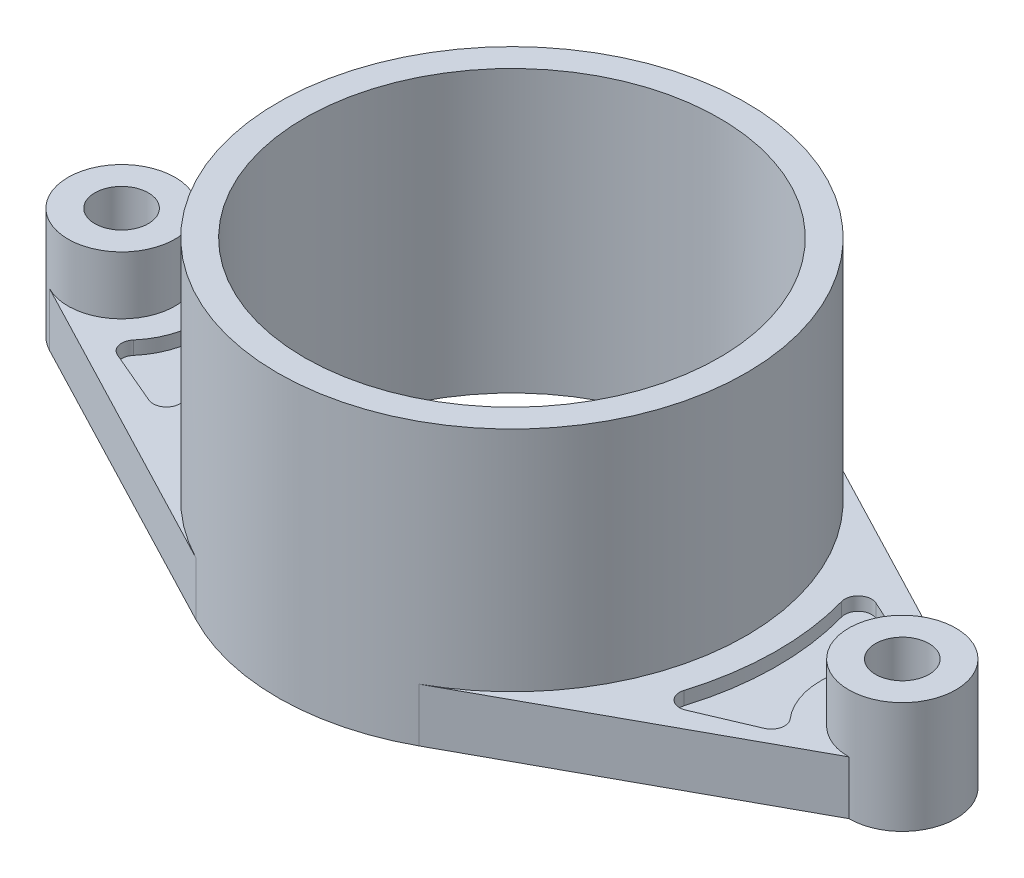
ISO-10303-21;
HEADER;
FILE_DESCRIPTION(('STEP AP214'),'2;1');
FILE_NAME('part.step','',(''),(''),'','','');
FILE_SCHEMA(('AUTOMOTIVE_DESIGN { 1 0 10303 214 1 1 1 1 }'));
ENDSEC;
DATA;
#1=APPLICATION_CONTEXT('core data for automotive mechanical design processes');
#2=APPLICATION_PROTOCOL_DEFINITION('international standard','automotive_design',2000,#1);
#3=PRODUCT_CONTEXT('',#1,'mechanical');
#4=PRODUCT('Part','Part','',(#3));
#5=PRODUCT_RELATED_PRODUCT_CATEGORY('part','',(#4));
#6=PRODUCT_DEFINITION_FORMATION('','',#4);
#7=PRODUCT_DEFINITION_CONTEXT('part definition',#1,'design');
#8=PRODUCT_DEFINITION('design','',#6,#7);
#9=PRODUCT_DEFINITION_SHAPE('','',#8);
#10=(LENGTH_UNIT() NAMED_UNIT(*) SI_UNIT(.MILLI.,.METRE.));
#11=(NAMED_UNIT(*) PLANE_ANGLE_UNIT() SI_UNIT($,.RADIAN.));
#12=(NAMED_UNIT(*) SI_UNIT($,.STERADIAN.) SOLID_ANGLE_UNIT());
#13=UNCERTAINTY_MEASURE_WITH_UNIT(LENGTH_MEASURE(1.E-05),#10,'distance_accuracy_value','');
#14=(GEOMETRIC_REPRESENTATION_CONTEXT(3) GLOBAL_UNCERTAINTY_ASSIGNED_CONTEXT((#13)) GLOBAL_UNIT_ASSIGNED_CONTEXT((#10,
#11,#12)) REPRESENTATION_CONTEXT('',''));
#15=CARTESIAN_POINT('',(0.,0.,0.));
#16=DIRECTION('',(0.,0.,1.));
#17=DIRECTION('',(1.,0.,0.));
#18=AXIS2_PLACEMENT_3D('',#15,#16,#17);
#19=CARTESIAN_POINT('',(0.,12.,0.));
#20=DIRECTION('',(0.,1.,0.));
#21=DIRECTION('',(0.,0.,1.));
#22=AXIS2_PLACEMENT_3D('',#19,#20,#21);
#23=PLANE('',#22);
#24=CARTESIAN_POINT('',(87.5,12.,0.));
#25=DIRECTION('',(0.,1.,0.));
#26=DIRECTION('',(0.,0.,1.));
#27=AXIS2_PLACEMENT_3D('',#24,#25,#26);
#28=CIRCLE('',#27,12.);
#29=CARTESIAN_POINT('',(93.0542857142854,12.,-10.6371946585583));
#30=VERTEX_POINT('',#29);
#31=CARTESIAN_POINT('',(87.5,12.,12.));
#32=VERTEX_POINT('',#31);
#33=EDGE_CURVE('E362',#30,#32,#28,.T.);
#34=ORIENTED_EDGE('',*,*,#33,.F.);
#35=DIRECTION('',(-0.886432888213266,0.,-0.462857142857154));
#36=VECTOR('',#35,1.);
#37=CARTESIAN_POINT('',(24.3000000000006,12.,-46.5377266311965));
#38=LINE('',#37,#36);
#39=CARTESIAN_POINT('',(24.3000000000006,12.,-46.5377266311965));
#40=VERTEX_POINT('',#39);
#41=EDGE_CURVE('E364',#30,#40,#38,.T.);
#42=ORIENTED_EDGE('',*,*,#41,.T.);
#43=CARTESIAN_POINT('',(0.,12.,0.));
#44=DIRECTION('',(0.,1.,0.));
#45=DIRECTION('',(0.,0.,1.));
#46=AXIS2_PLACEMENT_3D('',#43,#44,#45);
#47=CIRCLE('',#46,52.5);
#48=CARTESIAN_POINT('',(25.1823425044712,12.,46.0662525715681));
#49=VERTEX_POINT('',#48);
#50=EDGE_CURVE('E369',#49,#40,#47,.T.);
#51=ORIENTED_EDGE('',*,*,#50,.F.);
#52=DIRECTION('',(-0.877452429934631,0.,0.479663666751831));
#53=VECTOR('',#52,1.);
#54=CARTESIAN_POINT('',(25.1823425044711,12.,46.0662525715681));
#55=LINE('',#54,#53);
#56=EDGE_CURVE('E371',#32,#49,#55,.T.);
#57=ORIENTED_EDGE('',*,*,#56,.F.);
#58=EDGE_LOOP('',(#34,#42,#51,#57));
#59=FACE_BOUND('',#58,.T.);
#60=CARTESIAN_POINT('',(59.4229736389567,12.,-18.1878630690945));
#61=DIRECTION('',(0.,1.,0.));
#62=DIRECTION('',(0.,0.,-1.));
#63=AXIS2_PLACEMENT_3D('',#60,#61,#62);
#64=CIRCLE('',#63,3.);
#65=CARTESIAN_POINT('',(60.670465140095,12.,-20.9161894708631));
#66=VERTEX_POINT('',#65);
#67=CARTESIAN_POINT('',(56.5356423498588,12.,-17.3734196843239));
#68=VERTEX_POINT('',#67);
#69=EDGE_CURVE('E69',#66,#68,#64,.T.);
#70=ORIENTED_EDGE('',*,*,#69,.F.);
#71=DIRECTION('',(-0.90944213392287,0.,-0.415830500379442));
#72=VECTOR('',#71,1.);
#73=CARTESIAN_POINT('',(60.670465140095,12.,-20.9161894708631));
#74=LINE('',#73,#72);
#75=CARTESIAN_POINT('',(72.8322479303877,12.,-15.3553736316198));
#76=VERTEX_POINT('',#75);
#77=EDGE_CURVE('E278',#76,#66,#74,.T.);
#78=ORIENTED_EDGE('',*,*,#77,.F.);
#79=CARTESIAN_POINT('',(71.5847564292494,12.,-12.6270472298512));
#80=DIRECTION('',(0.,1.,0.));
#81=DIRECTION('',(0.,0.,-1.));
#82=AXIS2_PLACEMENT_3D('',#79,#80,#81);
#83=CIRCLE('',#82,3.);
#84=CARTESIAN_POINT('',(73.8195893160945,12.,-10.6256672139932));
#85=VERTEX_POINT('',#84);
#86=EDGE_CURVE('E318',#85,#76,#83,.T.);
#87=ORIENTED_EDGE('',*,*,#86,.F.);
#88=CARTESIAN_POINT('',(86.1725998126227,12.,0.436935492886657));
#89=DIRECTION('',(0.,-1.,0.));
#90=DIRECTION('',(0.,0.,1.));
#91=AXIS2_PLACEMENT_3D('',#88,#89,#90);
#92=CIRCLE('',#91,16.5824620300365);
#93=CARTESIAN_POINT('',(73.5829785567061,12.,11.2295016200955));
#94=VERTEX_POINT('',#93);
#95=EDGE_CURVE('E312',#94,#85,#92,.T.);
#96=ORIENTED_EDGE('',*,*,#95,.F.);
#97=CARTESIAN_POINT('',(71.3053394643122,12.,13.1820282306181));
#98=DIRECTION('',(0.,1.,0.));
#99=DIRECTION('',(0.,0.,-1.));
#100=AXIS2_PLACEMENT_3D('',#97,#98,#99);
#101=CIRCLE('',#100,3.);
#102=CARTESIAN_POINT('',(72.4819315608604,12.,15.941671511613));
#103=VERTEX_POINT('',#102);
#104=EDGE_CURVE('E315',#103,#94,#101,.T.);
#105=ORIENTED_EDGE('',*,*,#104,.F.);
#106=DIRECTION('',(0.919881093664966,0.,-0.392197365516071));
#107=VECTOR('',#106,1.);
#108=CARTESIAN_POINT('',(60.1771351937797,12.,21.1879025208334));
#109=LINE('',#108,#107);
#110=CARTESIAN_POINT('',(60.1771351937797,12.,21.1879025208334));
#111=VERTEX_POINT('',#110);
#112=EDGE_CURVE('E310',#111,#103,#109,.T.);
#113=ORIENTED_EDGE('',*,*,#112,.F.);
#114=CARTESIAN_POINT('',(59.0005430972315,12.,18.4282592398385));
#115=DIRECTION('',(0.,1.,0.));
#116=DIRECTION('',(0.,0.,-1.));
#117=AXIS2_PLACEMENT_3D('',#114,#115,#116);
#118=CIRCLE('',#117,3.);
#119=CARTESIAN_POINT('',(56.1327698280164,12.,17.5474207322928));
#120=VERTEX_POINT('',#119);
#121=EDGE_CURVE('E308',#120,#111,#118,.T.);
#122=ORIENTED_EDGE('',*,*,#121,.F.);
#123=CARTESIAN_POINT('',(-2.94003283636643,12.,-0.596830730682654));
#124=DIRECTION('',(0.,-1.,0.));
#125=DIRECTION('',(0.,0.,-1.));
#126=AXIS2_PLACEMENT_3D('',#123,#124,#125);
#127=CIRCLE('',#126,61.7965199325723);
#128=EDGE_CURVE('E305',#68,#120,#127,.T.);
#129=ORIENTED_EDGE('',*,*,#128,.F.);
#130=EDGE_LOOP('',(#70,#78,#87,#96,#105,#113,#122,#129));
#131=FACE_BOUND('',#130,.T.);
#132=ADVANCED_FACE('F41',(#59,#131),#23,.T.);
#133=CARTESIAN_POINT('',(0.,63.,0.));
#134=DIRECTION('',(0.,-1.,0.));
#135=DIRECTION('',(0.,0.,-1.));
#136=AXIS2_PLACEMENT_3D('',#133,#134,#135);
#137=CYLINDRICAL_SURFACE('',#136,52.5);
#138=ORIENTED_EDGE('',*,*,#50,.T.);
#139=DIRECTION('',(0.,-1.,0.));
#140=VECTOR('',#139,1.);
#141=CARTESIAN_POINT('',(24.3000000000006,12.,-46.5377266311965));
#142=LINE('',#141,#140);
#143=CARTESIAN_POINT('',(24.3000000000006,0.,-46.5377266311965));
#144=VERTEX_POINT('',#143);
#145=EDGE_CURVE('E383',#40,#144,#142,.T.);
#146=ORIENTED_EDGE('',*,*,#145,.T.);
#147=CARTESIAN_POINT('',(0.,0.,0.));
#148=DIRECTION('',(0.,1.,0.));
#149=DIRECTION('',(0.,0.,1.));
#150=AXIS2_PLACEMENT_3D('',#147,#148,#149);
#151=CIRCLE('',#150,52.5);
#152=CARTESIAN_POINT('',(-24.3000000000006,0.,-46.5377266311965));
#153=VERTEX_POINT('',#152);
#154=EDGE_CURVE('E418',#144,#153,#151,.T.);
#155=ORIENTED_EDGE('',*,*,#154,.T.);
#156=DIRECTION('',(0.,-1.,0.));
#157=VECTOR('',#156,1.);
#158=CARTESIAN_POINT('',(-24.3000000000006,12.,-46.5377266311965));
#159=LINE('',#158,#157);
#160=CARTESIAN_POINT('',(-24.3000000000006,12.,-46.5377266311965));
#161=VERTEX_POINT('',#160);
#162=EDGE_CURVE('E413',#161,#153,#159,.T.);
#163=ORIENTED_EDGE('',*,*,#162,.F.);
#164=CARTESIAN_POINT('',(0.,12.,0.));
#165=DIRECTION('',(0.,1.,0.));
#166=DIRECTION('',(0.,0.,1.));
#167=AXIS2_PLACEMENT_3D('',#164,#165,#166);
#168=CIRCLE('',#167,52.5);
#169=CARTESIAN_POINT('',(-24.3000000000006,12.,46.5377266311965));
#170=VERTEX_POINT('',#169);
#171=EDGE_CURVE('E388',#161,#170,#168,.T.);
#172=ORIENTED_EDGE('',*,*,#171,.T.);
#173=DIRECTION('',(0.,-1.,0.));
#174=VECTOR('',#173,1.);
#175=CARTESIAN_POINT('',(-24.3000000000006,12.,46.5377266311965));
#176=LINE('',#175,#174);
#177=CARTESIAN_POINT('',(-24.3000000000006,0.,46.5377266311965));
#178=VERTEX_POINT('',#177);
#179=EDGE_CURVE('E405',#170,#178,#176,.T.);
#180=ORIENTED_EDGE('',*,*,#179,.T.);
#181=CARTESIAN_POINT('',(25.1823425044712,0.,46.0662525715681));
#182=VERTEX_POINT('',#181);
#183=EDGE_CURVE('E49',#178,#182,#151,.T.);
#184=ORIENTED_EDGE('',*,*,#183,.T.);
#185=DIRECTION('',(0.,-1.,0.));
#186=VECTOR('',#185,1.);
#187=CARTESIAN_POINT('',(25.1823425044711,12.,46.0662525715681));
#188=LINE('',#187,#186);
#189=EDGE_CURVE('E381',#49,#182,#188,.T.);
#190=ORIENTED_EDGE('',*,*,#189,.F.);
#191=EDGE_LOOP('',(#138,#146,#155,#163,#172,#180,#184,#190));
#192=FACE_BOUND('',#191,.T.);
#193=CARTESIAN_POINT('',(0.,63.,0.));
#194=DIRECTION('',(0.,1.,0.));
#195=DIRECTION('',(0.,0.,1.));
#196=AXIS2_PLACEMENT_3D('',#193,#194,#195);
#197=CIRCLE('',#196,52.5);
#198=CARTESIAN_POINT('',(0.,63.,52.5));
#199=VERTEX_POINT('',#198);
#200=EDGE_CURVE('E11',#199,#199,#197,.T.);
#201=ORIENTED_EDGE('',*,*,#200,.F.);
#202=EDGE_LOOP('',(#201));
#203=FACE_BOUND('',#202,.T.);
#204=ADVANCED_FACE('F43',(#192,#203),#137,.T.);
#205=CARTESIAN_POINT('',(0.,63.,0.));
#206=DIRECTION('',(0.,1.,0.));
#207=DIRECTION('',(0.,0.,1.));
#208=AXIS2_PLACEMENT_3D('',#205,#206,#207);
#209=PLANE('',#208);
#210=CARTESIAN_POINT('',(0.,63.,0.));
#211=DIRECTION('',(0.,1.,0.));
#212=DIRECTION('',(0.,0.,1.));
#213=AXIS2_PLACEMENT_3D('',#210,#211,#212);
#214=CIRCLE('',#213,46.5);
#215=CARTESIAN_POINT('',(0.,63.,46.5));
#216=VERTEX_POINT('',#215);
#217=EDGE_CURVE('E343',#216,#216,#214,.T.);
#218=ORIENTED_EDGE('',*,*,#217,.F.);
#219=EDGE_LOOP('',(#218));
#220=FACE_BOUND('',#219,.T.);
#221=ORIENTED_EDGE('',*,*,#200,.T.);
#222=EDGE_LOOP('',(#221));
#223=FACE_BOUND('',#222,.T.);
#224=ADVANCED_FACE('F486',(#220,#223),#209,.T.);
#225=CARTESIAN_POINT('',(0.,0.,0.));
#226=DIRECTION('',(0.,1.,0.));
#227=DIRECTION('',(0.,0.,1.));
#228=AXIS2_PLACEMENT_3D('',#225,#226,#227);
#229=PLANE('',#228);
#230=CARTESIAN_POINT('',(-87.5,0.,0.));
#231=DIRECTION('',(0.,1.,0.));
#232=DIRECTION('',(0.,0.,1.));
#233=AXIS2_PLACEMENT_3D('',#230,#231,#232);
#234=CIRCLE('',#233,6.);
#235=CARTESIAN_POINT('',(-87.5,0.,6.));
#236=VERTEX_POINT('',#235);
#237=EDGE_CURVE('E339',#236,#236,#234,.T.);
#238=ORIENTED_EDGE('',*,*,#237,.T.);
#239=EDGE_LOOP('',(#238));
#240=FACE_BOUND('',#239,.T.);
#241=CARTESIAN_POINT('',(0.,0.,0.));
#242=DIRECTION('',(0.,1.,0.));
#243=DIRECTION('',(0.,0.,1.));
#244=AXIS2_PLACEMENT_3D('',#241,#242,#243);
#245=CIRCLE('',#244,46.5);
#246=CARTESIAN_POINT('',(0.,0.,46.5));
#247=VERTEX_POINT('',#246);
#248=EDGE_CURVE('E344',#247,#247,#245,.T.);
#249=ORIENTED_EDGE('',*,*,#248,.T.);
#250=EDGE_LOOP('',(#249));
#251=FACE_BOUND('',#250,.T.);
#252=CARTESIAN_POINT('',(87.5,0.,0.));
#253=DIRECTION('',(0.,1.,0.));
#254=DIRECTION('',(0.,0.,1.));
#255=AXIS2_PLACEMENT_3D('',#252,#253,#254);
#256=CIRCLE('',#255,6.);
#257=CARTESIAN_POINT('',(87.5,0.,6.));
#258=VERTEX_POINT('',#257);
#259=EDGE_CURVE('E262',#258,#258,#256,.T.);
#260=ORIENTED_EDGE('',*,*,#259,.T.);
#261=EDGE_LOOP('',(#260));
#262=FACE_BOUND('',#261,.T.);
#263=ORIENTED_EDGE('',*,*,#183,.F.);
#264=DIRECTION('',(0.886432888213266,0.,0.462857142857154));
#265=VECTOR('',#264,1.);
#266=CARTESIAN_POINT('',(-24.3000000000006,0.,46.5377266311965));
#267=LINE('',#266,#265);
#268=CARTESIAN_POINT('',(-93.0542857142854,0.,10.6371946585583));
#269=VERTEX_POINT('',#268);
#270=EDGE_CURVE('E395',#269,#178,#267,.T.);
#271=ORIENTED_EDGE('',*,*,#270,.F.);
#272=CARTESIAN_POINT('',(-87.5,0.,0.));
#273=DIRECTION('',(0.,1.,0.));
#274=DIRECTION('',(0.,0.,1.));
#275=AXIS2_PLACEMENT_3D('',#272,#273,#274);
#276=CIRCLE('',#275,12.);
#277=CARTESIAN_POINT('',(-93.0542857142854,0.,-10.6371946585583));
#278=VERTEX_POINT('',#277);
#279=EDGE_CURVE('E349',#278,#269,#276,.T.);
#280=ORIENTED_EDGE('',*,*,#279,.F.);
#281=DIRECTION('',(0.886432888213266,0.,-0.462857142857154));
#282=VECTOR('',#281,1.);
#283=CARTESIAN_POINT('',(-24.3000000000006,0.,-46.5377266311965));
#284=LINE('',#283,#282);
#285=EDGE_CURVE('E386',#278,#153,#284,.T.);
#286=ORIENTED_EDGE('',*,*,#285,.T.);
#287=ORIENTED_EDGE('',*,*,#154,.F.);
#288=DIRECTION('',(-0.886432888213266,0.,-0.462857142857154));
#289=VECTOR('',#288,1.);
#290=CARTESIAN_POINT('',(24.3000000000006,0.,-46.5377266311965));
#291=LINE('',#290,#289);
#292=CARTESIAN_POINT('',(93.0542857142854,0.,-10.6371946585583));
#293=VERTEX_POINT('',#292);
#294=EDGE_CURVE('E358',#293,#144,#291,.T.);
#295=ORIENTED_EDGE('',*,*,#294,.F.);
#296=CARTESIAN_POINT('',(87.5,0.,0.));
#297=DIRECTION('',(0.,1.,0.));
#298=DIRECTION('',(0.,0.,1.));
#299=AXIS2_PLACEMENT_3D('',#296,#297,#298);
#300=CIRCLE('',#299,12.);
#301=CARTESIAN_POINT('',(87.5,0.,11.9999999999991));
#302=VERTEX_POINT('',#301);
#303=EDGE_CURVE('E354',#302,#293,#300,.T.);
#304=ORIENTED_EDGE('',*,*,#303,.F.);
#305=DIRECTION('',(-0.877452429934631,0.,0.479663666751831));
#306=VECTOR('',#305,1.);
#307=CARTESIAN_POINT('',(25.1823425044711,0.,46.0662525715681));
#308=LINE('',#307,#306);
#309=EDGE_CURVE('E368',#302,#182,#308,.T.);
#310=ORIENTED_EDGE('',*,*,#309,.T.);
#311=EDGE_LOOP('',(#263,#271,#280,#286,#287,#295,#304,#310));
#312=FACE_BOUND('',#311,.T.);
#313=ADVANCED_FACE('F441',(#240,#251,#262,#312),#229,.F.);
#314=CARTESIAN_POINT('',(-24.3000000000006,12.,-46.5377266311965));
#315=DIRECTION('',(-0.462857142857154,0.,-0.886432888213266));
#316=DIRECTION('',(-0.886432888213266,0.,0.462857142857154));
#317=AXIS2_PLACEMENT_3D('',#314,#315,#316);
#318=PLANE('',#317);
#319=ORIENTED_EDGE('',*,*,#285,.F.);
#320=DIRECTION('',(0.,-1.,0.));
#321=VECTOR('',#320,1.);
#322=CARTESIAN_POINT('',(-93.0542857142854,12.,-10.6371946585583));
#323=LINE('',#322,#321);
#324=CARTESIAN_POINT('',(-93.0542857142854,12.,-10.6371946585583));
#325=VERTEX_POINT('',#324);
#326=EDGE_CURVE('E414',#325,#278,#323,.T.);
#327=ORIENTED_EDGE('',*,*,#326,.F.);
#328=DIRECTION('',(0.886432888213266,0.,-0.462857142857154));
#329=VECTOR('',#328,1.);
#330=CARTESIAN_POINT('',(-24.3000000000006,12.,-46.5377266311965));
#331=LINE('',#330,#329);
#332=EDGE_CURVE('E394',#325,#161,#331,.T.);
#333=ORIENTED_EDGE('',*,*,#332,.T.);
#334=ORIENTED_EDGE('',*,*,#162,.T.);
#335=EDGE_LOOP('',(#319,#327,#333,#334));
#336=FACE_BOUND('',#335,.T.);
#337=ADVANCED_FACE('F463',(#336),#318,.T.);
#338=CARTESIAN_POINT('',(-24.3000000000006,12.,46.5377266311965));
#339=DIRECTION('',(0.462857142857154,0.,-0.886432888213266));
#340=DIRECTION('',(-0.886432888213266,0.,-0.462857142857154));
#341=AXIS2_PLACEMENT_3D('',#338,#339,#340);
#342=PLANE('',#341);
#343=ORIENTED_EDGE('',*,*,#270,.T.);
#344=ORIENTED_EDGE('',*,*,#179,.F.);
#345=DIRECTION('',(0.886432888213266,0.,0.462857142857154));
#346=VECTOR('',#345,1.);
#347=CARTESIAN_POINT('',(-24.3000000000006,12.,46.5377266311965));
#348=LINE('',#347,#346);
#349=CARTESIAN_POINT('',(-93.0542857142854,12.,10.6371946585583));
#350=VERTEX_POINT('',#349);
#351=EDGE_CURVE('E398',#350,#170,#348,.T.);
#352=ORIENTED_EDGE('',*,*,#351,.F.);
#353=DIRECTION('',(0.,-1.,0.));
#354=VECTOR('',#353,1.);
#355=CARTESIAN_POINT('',(-93.0542857142854,12.,10.6371946585583));
#356=LINE('',#355,#354);
#357=EDGE_CURVE('E406',#350,#269,#356,.T.);
#358=ORIENTED_EDGE('',*,*,#357,.T.);
#359=EDGE_LOOP('',(#343,#344,#352,#358));
#360=FACE_BOUND('',#359,.T.);
#361=ADVANCED_FACE('F468',(#360),#342,.F.);
#362=CARTESIAN_POINT('',(0.,12.,0.));
#363=DIRECTION('',(0.,1.,0.));
#364=DIRECTION('',(0.,0.,1.));
#365=AXIS2_PLACEMENT_3D('',#362,#363,#364);
#366=PLANE('',#365);
#367=CARTESIAN_POINT('',(-71.3053394643122,12.,13.1820282306181));
#368=DIRECTION('',(0.,1.,0.));
#369=DIRECTION('',(0.,0.,1.));
#370=AXIS2_PLACEMENT_3D('',#367,#368,#369);
#371=CIRCLE('',#370,3.);
#372=CARTESIAN_POINT('',(-73.5829785567061,12.,11.2295016200955));
#373=VERTEX_POINT('',#372);
#374=CARTESIAN_POINT('',(-72.4819315608604,12.,15.941671511613));
#375=VERTEX_POINT('',#374);
#376=EDGE_CURVE('E59',#373,#375,#371,.T.);
#377=ORIENTED_EDGE('',*,*,#376,.F.);
#378=CARTESIAN_POINT('',(-86.1725998126227,12.,0.436935492886657));
#379=DIRECTION('',(0.,-1.,0.));
#380=DIRECTION('',(0.,0.,-1.));
#381=AXIS2_PLACEMENT_3D('',#378,#379,#380);
#382=CIRCLE('',#381,16.5824620300365);
#383=CARTESIAN_POINT('',(-73.8195893160945,12.,-10.6256672139932));
#384=VERTEX_POINT('',#383);
#385=EDGE_CURVE('E223',#384,#373,#382,.T.);
#386=ORIENTED_EDGE('',*,*,#385,.F.);
#387=CARTESIAN_POINT('',(-71.5847564292494,12.,-12.6270472298512));
#388=DIRECTION('',(0.,1.,0.));
#389=DIRECTION('',(0.,0.,1.));
#390=AXIS2_PLACEMENT_3D('',#387,#388,#389);
#391=CIRCLE('',#390,3.);
#392=CARTESIAN_POINT('',(-72.8322479303877,12.,-15.3553736316198));
#393=VERTEX_POINT('',#392);
#394=EDGE_CURVE('E230',#393,#384,#391,.T.);
#395=ORIENTED_EDGE('',*,*,#394,.F.);
#396=DIRECTION('',(-0.90944213392287,0.,0.415830500379442));
#397=VECTOR('',#396,1.);
#398=CARTESIAN_POINT('',(-60.670465140095,12.,-20.9161894708631));
#399=LINE('',#398,#397);
#400=CARTESIAN_POINT('',(-60.670465140095,12.,-20.9161894708631));
#401=VERTEX_POINT('',#400);
#402=EDGE_CURVE('E260',#401,#393,#399,.T.);
#403=ORIENTED_EDGE('',*,*,#402,.F.);
#404=CARTESIAN_POINT('',(-59.4229736389567,12.,-18.1878630690945));
#405=DIRECTION('',(0.,1.,0.));
#406=DIRECTION('',(0.,0.,1.));
#407=AXIS2_PLACEMENT_3D('',#404,#405,#406);
#408=CIRCLE('',#407,3.);
#409=CARTESIAN_POINT('',(-56.5356423498588,12.,-17.3734196843239));
#410=VERTEX_POINT('',#409);
#411=EDGE_CURVE('E255',#410,#401,#408,.T.);
#412=ORIENTED_EDGE('',*,*,#411,.F.);
#413=CARTESIAN_POINT('',(2.94003283636643,12.,-0.596830730682654));
#414=DIRECTION('',(0.,-1.,0.));
#415=DIRECTION('',(0.,0.,1.));
#416=AXIS2_PLACEMENT_3D('',#413,#414,#415);
#417=CIRCLE('',#416,61.7965199325723);
#418=CARTESIAN_POINT('',(-56.1327698280164,12.,17.5474207322928));
#419=VERTEX_POINT('',#418);
#420=EDGE_CURVE('E253',#419,#410,#417,.T.);
#421=ORIENTED_EDGE('',*,*,#420,.F.);
#422=CARTESIAN_POINT('',(-59.0005430972315,12.,18.4282592398385));
#423=DIRECTION('',(0.,1.,0.));
#424=DIRECTION('',(0.,0.,1.));
#425=AXIS2_PLACEMENT_3D('',#422,#423,#424);
#426=CIRCLE('',#425,2.99999999999997);
#427=CARTESIAN_POINT('',(-60.1771351937798,12.,21.1879025208334));
#428=VERTEX_POINT('',#427);
#429=EDGE_CURVE('E250',#428,#419,#426,.T.);
#430=ORIENTED_EDGE('',*,*,#429,.F.);
#431=DIRECTION('',(0.919881093664967,0.,0.392197365516067));
#432=VECTOR('',#431,1.);
#433=CARTESIAN_POINT('',(-60.1771351937797,12.,21.1879025208334));
#434=LINE('',#433,#432);
#435=EDGE_CURVE('E243',#375,#428,#434,.T.);
#436=ORIENTED_EDGE('',*,*,#435,.F.);
#437=EDGE_LOOP('',(#377,#386,#395,#403,#412,#421,#430,#436));
#438=FACE_BOUND('',#437,.T.);
#439=ORIENTED_EDGE('',*,*,#171,.F.);
#440=ORIENTED_EDGE('',*,*,#332,.F.);
#441=CARTESIAN_POINT('',(-87.5,12.,0.));
#442=DIRECTION('',(0.,1.,0.));
#443=DIRECTION('',(0.,0.,1.));
#444=AXIS2_PLACEMENT_3D('',#441,#442,#443);
#445=CIRCLE('',#444,12.);
#446=EDGE_CURVE('E399',#350,#325,#445,.T.);
#447=ORIENTED_EDGE('',*,*,#446,.F.);
#448=ORIENTED_EDGE('',*,*,#351,.T.);
#449=EDGE_LOOP('',(#439,#440,#447,#448));
#450=FACE_BOUND('',#449,.T.);
#451=ADVANCED_FACE('F470',(#438,#450),#366,.T.);
#452=CARTESIAN_POINT('',(24.3000000000006,12.,-46.5377266311965));
#453=DIRECTION('',(-0.462857142857154,0.,0.886432888213266));
#454=DIRECTION('',(0.886432888213266,0.,0.462857142857154));
#455=AXIS2_PLACEMENT_3D('',#452,#453,#454);
#456=PLANE('',#455);
#457=ORIENTED_EDGE('',*,*,#294,.T.);
#458=ORIENTED_EDGE('',*,*,#145,.F.);
#459=ORIENTED_EDGE('',*,*,#41,.F.);
#460=DIRECTION('',(0.,-1.,0.));
#461=VECTOR('',#460,1.);
#462=CARTESIAN_POINT('',(93.0542857142854,12.,-10.6371946585583));
#463=LINE('',#462,#461);
#464=EDGE_CURVE('E390',#30,#293,#463,.T.);
#465=ORIENTED_EDGE('',*,*,#464,.T.);
#466=EDGE_LOOP('',(#457,#458,#459,#465));
#467=FACE_BOUND('',#466,.T.);
#468=ADVANCED_FACE('F449',(#467),#456,.F.);
#469=CARTESIAN_POINT('',(25.1823425044711,12.,46.0662525715681));
#470=DIRECTION('',(0.479663666751831,0.,0.877452429934631));
#471=DIRECTION('',(0.877452429934631,0.,-0.479663666751831));
#472=AXIS2_PLACEMENT_3D('',#469,#470,#471);
#473=PLANE('',#472);
#474=ORIENTED_EDGE('',*,*,#309,.F.);
#475=DIRECTION('',(0.,-1.,0.));
#476=VECTOR('',#475,1.);
#477=CARTESIAN_POINT('',(87.5,12.,11.9999999999991));
#478=LINE('',#477,#476);
#479=EDGE_CURVE('E372',#32,#302,#478,.T.);
#480=ORIENTED_EDGE('',*,*,#479,.F.);
#481=ORIENTED_EDGE('',*,*,#56,.T.);
#482=ORIENTED_EDGE('',*,*,#189,.T.);
#483=EDGE_LOOP('',(#474,#480,#481,#482));
#484=FACE_BOUND('',#483,.T.);
#485=ADVANCED_FACE('F440',(#484),#473,.T.);
#486=CARTESIAN_POINT('',(87.5,25.,0.));
#487=DIRECTION('',(0.,-1.,0.));
#488=DIRECTION('',(0.,0.,-1.));
#489=AXIS2_PLACEMENT_3D('',#486,#487,#488);
#490=CYLINDRICAL_SURFACE('',#489,12.);
#491=CARTESIAN_POINT('',(87.5,25.,0.));
#492=DIRECTION('',(0.,1.,0.));
#493=DIRECTION('',(0.,0.,1.));
#494=AXIS2_PLACEMENT_3D('',#491,#492,#493);
#495=CIRCLE('',#494,12.);
#496=CARTESIAN_POINT('',(87.5,25.,12.));
#497=VERTEX_POINT('',#496);
#498=EDGE_CURVE('E359',#497,#497,#495,.T.);
#499=ORIENTED_EDGE('',*,*,#498,.F.);
#500=EDGE_LOOP('',(#499));
#501=FACE_BOUND('',#500,.T.);
#502=ORIENTED_EDGE('',*,*,#303,.T.);
#503=ORIENTED_EDGE('',*,*,#464,.F.);
#504=ORIENTED_EDGE('',*,*,#33,.T.);
#505=ORIENTED_EDGE('',*,*,#479,.T.);
#506=EDGE_LOOP('',(#502,#503,#504,#505));
#507=FACE_BOUND('',#506,.T.);
#508=ADVANCED_FACE('F431',(#501,#507),#490,.T.);
#509=CARTESIAN_POINT('',(0.,25.,0.));
#510=DIRECTION('',(0.,1.,0.));
#511=DIRECTION('',(0.,0.,1.));
#512=AXIS2_PLACEMENT_3D('',#509,#510,#511);
#513=PLANE('',#512);
#514=CARTESIAN_POINT('',(87.5,25.,0.));
#515=DIRECTION('',(0.,1.,0.));
#516=DIRECTION('',(0.,0.,1.));
#517=AXIS2_PLACEMENT_3D('',#514,#515,#516);
#518=CIRCLE('',#517,6.);
#519=CARTESIAN_POINT('',(87.5,25.,6.));
#520=VERTEX_POINT('',#519);
#521=EDGE_CURVE('E44',#520,#520,#518,.T.);
#522=ORIENTED_EDGE('',*,*,#521,.F.);
#523=EDGE_LOOP('',(#522));
#524=FACE_BOUND('',#523,.T.);
#525=ORIENTED_EDGE('',*,*,#498,.T.);
#526=EDGE_LOOP('',(#525));
#527=FACE_BOUND('',#526,.T.);
#528=ADVANCED_FACE('F430',(#524,#527),#513,.T.);
#529=CARTESIAN_POINT('',(-87.5,25.,0.));
#530=DIRECTION('',(0.,-1.,0.));
#531=DIRECTION('',(0.,0.,-1.));
#532=AXIS2_PLACEMENT_3D('',#529,#530,#531);
#533=CYLINDRICAL_SURFACE('',#532,12.);
#534=ORIENTED_EDGE('',*,*,#326,.T.);
#535=ORIENTED_EDGE('',*,*,#279,.T.);
#536=ORIENTED_EDGE('',*,*,#357,.F.);
#537=ORIENTED_EDGE('',*,*,#446,.T.);
#538=EDGE_LOOP('',(#534,#535,#536,#537));
#539=FACE_BOUND('',#538,.T.);
#540=CARTESIAN_POINT('',(-87.5,25.,0.));
#541=DIRECTION('',(0.,1.,0.));
#542=DIRECTION('',(0.,0.,1.));
#543=AXIS2_PLACEMENT_3D('',#540,#541,#542);
#544=CIRCLE('',#543,12.);
#545=CARTESIAN_POINT('',(-87.5,25.,12.));
#546=VERTEX_POINT('',#545);
#547=EDGE_CURVE('E355',#546,#546,#544,.T.);
#548=ORIENTED_EDGE('',*,*,#547,.F.);
#549=EDGE_LOOP('',(#548));
#550=FACE_BOUND('',#549,.T.);
#551=ADVANCED_FACE('F429',(#539,#550),#533,.T.);
#552=CARTESIAN_POINT('',(-87.5,25.,0.));
#553=DIRECTION('',(0.,1.,0.));
#554=DIRECTION('',(0.,0.,1.));
#555=AXIS2_PLACEMENT_3D('',#552,#553,#554);
#556=PLANE('',#555);
#557=CARTESIAN_POINT('',(-87.5,25.,0.));
#558=DIRECTION('',(0.,1.,0.));
#559=DIRECTION('',(0.,0.,1.));
#560=AXIS2_PLACEMENT_3D('',#557,#558,#559);
#561=CIRCLE('',#560,6.);
#562=CARTESIAN_POINT('',(-87.5,25.,6.));
#563=VERTEX_POINT('',#562);
#564=EDGE_CURVE('E338',#563,#563,#561,.T.);
#565=ORIENTED_EDGE('',*,*,#564,.F.);
#566=EDGE_LOOP('',(#565));
#567=FACE_BOUND('',#566,.T.);
#568=ORIENTED_EDGE('',*,*,#547,.T.);
#569=EDGE_LOOP('',(#568));
#570=FACE_BOUND('',#569,.T.);
#571=ADVANCED_FACE('F511',(#567,#570),#556,.T.);
#572=CARTESIAN_POINT('',(-87.5,0.,0.));
#573=DIRECTION('',(0.,1.,0.));
#574=DIRECTION('',(0.,0.,1.));
#575=AXIS2_PLACEMENT_3D('',#572,#573,#574);
#576=CYLINDRICAL_SURFACE('',#575,6.);
#577=ORIENTED_EDGE('',*,*,#564,.T.);
#578=EDGE_LOOP('',(#577));
#579=FACE_BOUND('',#578,.T.);
#580=ORIENTED_EDGE('',*,*,#237,.F.);
#581=EDGE_LOOP('',(#580));
#582=FACE_BOUND('',#581,.T.);
#583=ADVANCED_FACE('F537',(#579,#582),#576,.F.);
#584=CARTESIAN_POINT('',(87.5,0.,0.));
#585=DIRECTION('',(0.,1.,0.));
#586=DIRECTION('',(0.,0.,1.));
#587=AXIS2_PLACEMENT_3D('',#584,#585,#586);
#588=CYLINDRICAL_SURFACE('',#587,6.);
#589=ORIENTED_EDGE('',*,*,#521,.T.);
#590=EDGE_LOOP('',(#589));
#591=FACE_BOUND('',#590,.T.);
#592=ORIENTED_EDGE('',*,*,#259,.F.);
#593=EDGE_LOOP('',(#592));
#594=FACE_BOUND('',#593,.T.);
#595=ADVANCED_FACE('F424',(#591,#594),#588,.F.);
#596=CARTESIAN_POINT('',(0.,0.,0.));
#597=DIRECTION('',(0.,1.,0.));
#598=DIRECTION('',(0.,0.,1.));
#599=AXIS2_PLACEMENT_3D('',#596,#597,#598);
#600=CYLINDRICAL_SURFACE('',#599,46.5);
#601=ORIENTED_EDGE('',*,*,#248,.F.);
#602=EDGE_LOOP('',(#601));
#603=FACE_BOUND('',#602,.T.);
#604=ORIENTED_EDGE('',*,*,#217,.T.);
#605=EDGE_LOOP('',(#604));
#606=FACE_BOUND('',#605,.T.);
#607=ADVANCED_FACE('F551',(#603,#606),#600,.F.);
#608=CARTESIAN_POINT('',(59.4229736389567,9.,-18.1878630690945));
#609=DIRECTION('',(0.,1.,0.));
#610=DIRECTION('',(0.,0.,1.));
#611=AXIS2_PLACEMENT_3D('',#608,#609,#610);
#612=CYLINDRICAL_SURFACE('',#611,3.);
#613=ORIENTED_EDGE('',*,*,#69,.T.);
#614=DIRECTION('',(0.,1.,0.));
#615=VECTOR('',#614,1.);
#616=CARTESIAN_POINT('',(56.5356423498588,9.,-17.3734196843239));
#617=LINE('',#616,#615);
#618=CARTESIAN_POINT('',(56.5356423498588,9.,-17.3734196843239));
#619=VERTEX_POINT('',#618);
#620=EDGE_CURVE('E304',#619,#68,#617,.T.);
#621=ORIENTED_EDGE('',*,*,#620,.F.);
#622=CARTESIAN_POINT('',(59.4229736389567,9.,-18.1878630690945));
#623=DIRECTION('',(0.,1.,0.));
#624=DIRECTION('',(0.,0.,-1.));
#625=AXIS2_PLACEMENT_3D('',#622,#623,#624);
#626=CIRCLE('',#625,3.);
#627=CARTESIAN_POINT('',(60.670465140095,9.,-20.9161894708631));
#628=VERTEX_POINT('',#627);
#629=EDGE_CURVE('E277',#628,#619,#626,.T.);
#630=ORIENTED_EDGE('',*,*,#629,.F.);
#631=DIRECTION('',(0.,1.,0.));
#632=VECTOR('',#631,1.);
#633=CARTESIAN_POINT('',(60.670465140095,9.,-20.9161894708631));
#634=LINE('',#633,#632);
#635=EDGE_CURVE('E249',#628,#66,#634,.T.);
#636=ORIENTED_EDGE('',*,*,#635,.T.);
#637=EDGE_LOOP('',(#613,#621,#630,#636));
#638=FACE_BOUND('',#637,.T.);
#639=ADVANCED_FACE('F564',(#638),#612,.F.);
#640=CARTESIAN_POINT('',(60.670465140095,9.,-20.9161894708631));
#641=DIRECTION('',(0.415830500379442,0.,-0.90944213392287));
#642=DIRECTION('',(-0.90944213392287,0.,-0.415830500379442));
#643=AXIS2_PLACEMENT_3D('',#640,#641,#642);
#644=PLANE('',#643);
#645=ORIENTED_EDGE('',*,*,#77,.T.);
#646=ORIENTED_EDGE('',*,*,#635,.F.);
#647=DIRECTION('',(-0.90944213392287,0.,-0.415830500379442));
#648=VECTOR('',#647,1.);
#649=CARTESIAN_POINT('',(60.670465140095,9.,-20.9161894708631));
#650=LINE('',#649,#648);
#651=CARTESIAN_POINT('',(72.8322479303877,9.,-15.3553736316198));
#652=VERTEX_POINT('',#651);
#653=EDGE_CURVE('E300',#652,#628,#650,.T.);
#654=ORIENTED_EDGE('',*,*,#653,.F.);
#655=DIRECTION('',(0.,1.,0.));
#656=VECTOR('',#655,1.);
#657=CARTESIAN_POINT('',(72.8322479303877,9.,-15.3553736316198));
#658=LINE('',#657,#656);
#659=EDGE_CURVE('E322',#652,#76,#658,.T.);
#660=ORIENTED_EDGE('',*,*,#659,.T.);
#661=EDGE_LOOP('',(#645,#646,#654,#660));
#662=FACE_BOUND('',#661,.T.);
#663=ADVANCED_FACE('F580',(#662),#644,.F.);
#664=CARTESIAN_POINT('',(71.5847564292494,9.,-12.6270472298512));
#665=DIRECTION('',(0.,1.,0.));
#666=DIRECTION('',(0.,0.,1.));
#667=AXIS2_PLACEMENT_3D('',#664,#665,#666);
#668=CYLINDRICAL_SURFACE('',#667,3.);
#669=ORIENTED_EDGE('',*,*,#86,.T.);
#670=ORIENTED_EDGE('',*,*,#659,.F.);
#671=CARTESIAN_POINT('',(71.5847564292494,9.,-12.6270472298512));
#672=DIRECTION('',(0.,1.,0.));
#673=DIRECTION('',(0.,0.,-1.));
#674=AXIS2_PLACEMENT_3D('',#671,#672,#673);
#675=CIRCLE('',#674,3.);
#676=CARTESIAN_POINT('',(73.8195893160945,9.,-10.6256672139932));
#677=VERTEX_POINT('',#676);
#678=EDGE_CURVE('E293',#677,#652,#675,.T.);
#679=ORIENTED_EDGE('',*,*,#678,.F.);
#680=DIRECTION('',(0.,1.,0.));
#681=VECTOR('',#680,1.);
#682=CARTESIAN_POINT('',(73.8195893160945,9.,-10.6256672139932));
#683=LINE('',#682,#681);
#684=EDGE_CURVE('E326',#677,#85,#683,.T.);
#685=ORIENTED_EDGE('',*,*,#684,.T.);
#686=EDGE_LOOP('',(#669,#670,#679,#685));
#687=FACE_BOUND('',#686,.T.);
#688=ADVANCED_FACE('F590',(#687),#668,.F.);
#689=CARTESIAN_POINT('',(86.1725998126227,9.,0.436935492886657));
#690=DIRECTION('',(0.,1.,0.));
#691=DIRECTION('',(0.,0.,1.));
#692=AXIS2_PLACEMENT_3D('',#689,#690,#691);
#693=CYLINDRICAL_SURFACE('',#692,16.5824620300365);
#694=ORIENTED_EDGE('',*,*,#95,.T.);
#695=ORIENTED_EDGE('',*,*,#684,.F.);
#696=CARTESIAN_POINT('',(86.1725998126227,9.,0.436935492886657));
#697=DIRECTION('',(0.,-1.,0.));
#698=DIRECTION('',(0.,0.,1.));
#699=AXIS2_PLACEMENT_3D('',#696,#697,#698);
#700=CIRCLE('',#699,16.5824620300365);
#701=CARTESIAN_POINT('',(73.5829785567061,9.,11.2295016200955));
#702=VERTEX_POINT('',#701);
#703=EDGE_CURVE('E295',#702,#677,#700,.T.);
#704=ORIENTED_EDGE('',*,*,#703,.F.);
#705=DIRECTION('',(0.,1.,0.));
#706=VECTOR('',#705,1.);
#707=CARTESIAN_POINT('',(73.5829785567061,9.,11.2295016200955));
#708=LINE('',#707,#706);
#709=EDGE_CURVE('E327',#702,#94,#708,.T.);
#710=ORIENTED_EDGE('',*,*,#709,.T.);
#711=EDGE_LOOP('',(#694,#695,#704,#710));
#712=FACE_BOUND('',#711,.T.);
#713=ADVANCED_FACE('F600',(#712),#693,.T.);
#714=CARTESIAN_POINT('',(71.3053394643122,9.,13.1820282306181));
#715=DIRECTION('',(0.,1.,0.));
#716=DIRECTION('',(0.,0.,1.));
#717=AXIS2_PLACEMENT_3D('',#714,#715,#716);
#718=CYLINDRICAL_SURFACE('',#717,3.);
#719=ORIENTED_EDGE('',*,*,#104,.T.);
#720=ORIENTED_EDGE('',*,*,#709,.F.);
#721=CARTESIAN_POINT('',(71.3053394643122,9.,13.1820282306181));
#722=DIRECTION('',(0.,1.,0.));
#723=DIRECTION('',(0.,0.,-1.));
#724=AXIS2_PLACEMENT_3D('',#721,#722,#723);
#725=CIRCLE('',#724,3.);
#726=CARTESIAN_POINT('',(72.4819315608604,9.,15.941671511613));
#727=VERTEX_POINT('',#726);
#728=EDGE_CURVE('E288',#727,#702,#725,.T.);
#729=ORIENTED_EDGE('',*,*,#728,.F.);
#730=DIRECTION('',(0.,1.,0.));
#731=VECTOR('',#730,1.);
#732=CARTESIAN_POINT('',(72.4819315608604,9.,15.941671511613));
#733=LINE('',#732,#731);
#734=EDGE_CURVE('E329',#727,#103,#733,.T.);
#735=ORIENTED_EDGE('',*,*,#734,.T.);
#736=EDGE_LOOP('',(#719,#720,#729,#735));
#737=FACE_BOUND('',#736,.T.);
#738=ADVANCED_FACE('F610',(#737),#718,.F.);
#739=CARTESIAN_POINT('',(60.1771351937797,9.,21.1879025208334));
#740=DIRECTION('',(0.392197365516071,0.,0.919881093664966));
#741=DIRECTION('',(0.919881093664966,0.,-0.392197365516071));
#742=AXIS2_PLACEMENT_3D('',#739,#740,#741);
#743=PLANE('',#742);
#744=ORIENTED_EDGE('',*,*,#112,.T.);
#745=ORIENTED_EDGE('',*,*,#734,.F.);
#746=DIRECTION('',(0.919881093664966,0.,-0.392197365516071));
#747=VECTOR('',#746,1.);
#748=CARTESIAN_POINT('',(60.1771351937797,9.,21.1879025208334));
#749=LINE('',#748,#747);
#750=CARTESIAN_POINT('',(60.1771351937797,9.,21.1879025208334));
#751=VERTEX_POINT('',#750);
#752=EDGE_CURVE('E289',#751,#727,#749,.T.);
#753=ORIENTED_EDGE('',*,*,#752,.F.);
#754=DIRECTION('',(0.,1.,0.));
#755=VECTOR('',#754,1.);
#756=CARTESIAN_POINT('',(60.1771351937797,9.,21.1879025208334));
#757=LINE('',#756,#755);
#758=EDGE_CURVE('E335',#751,#111,#757,.T.);
#759=ORIENTED_EDGE('',*,*,#758,.T.);
#760=EDGE_LOOP('',(#744,#745,#753,#759));
#761=FACE_BOUND('',#760,.T.);
#762=ADVANCED_FACE('F616',(#761),#743,.F.);
#763=CARTESIAN_POINT('',(59.0005430972315,9.,18.4282592398385));
#764=DIRECTION('',(0.,1.,0.));
#765=DIRECTION('',(0.,0.,1.));
#766=AXIS2_PLACEMENT_3D('',#763,#764,#765);
#767=CYLINDRICAL_SURFACE('',#766,3.);
#768=ORIENTED_EDGE('',*,*,#121,.T.);
#769=ORIENTED_EDGE('',*,*,#758,.F.);
#770=CARTESIAN_POINT('',(59.0005430972315,9.,18.4282592398385));
#771=DIRECTION('',(0.,1.,0.));
#772=DIRECTION('',(0.,0.,-1.));
#773=AXIS2_PLACEMENT_3D('',#770,#771,#772);
#774=CIRCLE('',#773,3.);
#775=CARTESIAN_POINT('',(56.1327698280164,9.,17.5474207322928));
#776=VERTEX_POINT('',#775);
#777=EDGE_CURVE('E285',#776,#751,#774,.T.);
#778=ORIENTED_EDGE('',*,*,#777,.F.);
#779=DIRECTION('',(0.,1.,0.));
#780=VECTOR('',#779,1.);
#781=CARTESIAN_POINT('',(56.1327698280164,9.,17.5474207322928));
#782=LINE('',#781,#780);
#783=EDGE_CURVE('E331',#776,#120,#782,.T.);
#784=ORIENTED_EDGE('',*,*,#783,.T.);
#785=EDGE_LOOP('',(#768,#769,#778,#784));
#786=FACE_BOUND('',#785,.T.);
#787=ADVANCED_FACE('F629',(#786),#767,.F.);
#788=CARTESIAN_POINT('',(-2.94003283636643,9.,-0.596830730682654));
#789=DIRECTION('',(0.,1.,0.));
#790=DIRECTION('',(0.,0.,1.));
#791=AXIS2_PLACEMENT_3D('',#788,#789,#790);
#792=CYLINDRICAL_SURFACE('',#791,61.7965199325723);
#793=ORIENTED_EDGE('',*,*,#128,.T.);
#794=ORIENTED_EDGE('',*,*,#783,.F.);
#795=CARTESIAN_POINT('',(-2.94003283636643,9.,-0.596830730682654));
#796=DIRECTION('',(0.,-1.,0.));
#797=DIRECTION('',(0.,0.,-1.));
#798=AXIS2_PLACEMENT_3D('',#795,#796,#797);
#799=CIRCLE('',#798,61.7965199325723);
#800=EDGE_CURVE('E276',#619,#776,#799,.T.);
#801=ORIENTED_EDGE('',*,*,#800,.F.);
#802=ORIENTED_EDGE('',*,*,#620,.T.);
#803=EDGE_LOOP('',(#793,#794,#801,#802));
#804=FACE_BOUND('',#803,.T.);
#805=ADVANCED_FACE('F637',(#804),#792,.T.);
#806=CARTESIAN_POINT('',(59.4229736389567,9.,-18.1878630690945));
#807=DIRECTION('',(0.,-1.,0.));
#808=DIRECTION('',(0.,0.,-1.));
#809=AXIS2_PLACEMENT_3D('',#806,#807,#808);
#810=PLANE('',#809);
#811=ORIENTED_EDGE('',*,*,#629,.T.);
#812=ORIENTED_EDGE('',*,*,#800,.T.);
#813=ORIENTED_EDGE('',*,*,#777,.T.);
#814=ORIENTED_EDGE('',*,*,#752,.T.);
#815=ORIENTED_EDGE('',*,*,#728,.T.);
#816=ORIENTED_EDGE('',*,*,#703,.T.);
#817=ORIENTED_EDGE('',*,*,#678,.T.);
#818=ORIENTED_EDGE('',*,*,#653,.T.);
#819=EDGE_LOOP('',(#811,#812,#813,#814,#815,#816,#817,#818));
#820=FACE_BOUND('',#819,.T.);
#821=ADVANCED_FACE('F650',(#820),#810,.F.);
#822=CARTESIAN_POINT('',(-71.3053394643122,9.,13.1820282306181));
#823=DIRECTION('',(0.,1.,0.));
#824=DIRECTION('',(0.,0.,1.));
#825=AXIS2_PLACEMENT_3D('',#822,#823,#824);
#826=CYLINDRICAL_SURFACE('',#825,3.);
#827=ORIENTED_EDGE('',*,*,#376,.T.);
#828=DIRECTION('',(0.,1.,0.));
#829=VECTOR('',#828,1.);
#830=CARTESIAN_POINT('',(-72.4819315608604,9.,15.941671511613));
#831=LINE('',#830,#829);
#832=CARTESIAN_POINT('',(-72.4819315608604,9.,15.941671511613));
#833=VERTEX_POINT('',#832);
#834=EDGE_CURVE('E205',#833,#375,#831,.T.);
#835=ORIENTED_EDGE('',*,*,#834,.F.);
#836=CARTESIAN_POINT('',(-71.3053394643122,9.,13.1820282306181));
#837=DIRECTION('',(0.,1.,0.));
#838=DIRECTION('',(0.,0.,1.));
#839=AXIS2_PLACEMENT_3D('',#836,#837,#838);
#840=CIRCLE('',#839,3.);
#841=CARTESIAN_POINT('',(-73.5829785567061,9.,11.2295016200955));
#842=VERTEX_POINT('',#841);
#843=EDGE_CURVE('E206',#842,#833,#840,.T.);
#844=ORIENTED_EDGE('',*,*,#843,.F.);
#845=DIRECTION('',(0.,1.,0.));
#846=VECTOR('',#845,1.);
#847=CARTESIAN_POINT('',(-73.5829785567061,9.,11.2295016200955));
#848=LINE('',#847,#846);
#849=EDGE_CURVE('E265',#842,#373,#848,.T.);
#850=ORIENTED_EDGE('',*,*,#849,.T.);
#851=EDGE_LOOP('',(#827,#835,#844,#850));
#852=FACE_BOUND('',#851,.T.);
#853=ADVANCED_FACE('F204',(#852),#826,.F.);
#854=CARTESIAN_POINT('',(-86.1725998126227,9.,0.436935492886657));
#855=DIRECTION('',(0.,1.,0.));
#856=DIRECTION('',(0.,0.,1.));
#857=AXIS2_PLACEMENT_3D('',#854,#855,#856);
#858=CYLINDRICAL_SURFACE('',#857,16.5824620300365);
#859=ORIENTED_EDGE('',*,*,#385,.T.);
#860=ORIENTED_EDGE('',*,*,#849,.F.);
#861=CARTESIAN_POINT('',(-86.1725998126227,9.,0.436935492886657));
#862=DIRECTION('',(0.,-1.,0.));
#863=DIRECTION('',(0.,0.,-1.));
#864=AXIS2_PLACEMENT_3D('',#861,#862,#863);
#865=CIRCLE('',#864,16.5824620300365);
#866=CARTESIAN_POINT('',(-73.8195893160945,9.,-10.6256672139932));
#867=VERTEX_POINT('',#866);
#868=EDGE_CURVE('E215',#867,#842,#865,.T.);
#869=ORIENTED_EDGE('',*,*,#868,.F.);
#870=DIRECTION('',(0.,1.,0.));
#871=VECTOR('',#870,1.);
#872=CARTESIAN_POINT('',(-73.8195893160945,9.,-10.6256672139932));
#873=LINE('',#872,#871);
#874=EDGE_CURVE('E264',#867,#384,#873,.T.);
#875=ORIENTED_EDGE('',*,*,#874,.T.);
#876=EDGE_LOOP('',(#859,#860,#869,#875));
#877=FACE_BOUND('',#876,.T.);
#878=ADVANCED_FACE('F667',(#877),#858,.T.);
#879=CARTESIAN_POINT('',(-71.5847564292494,9.,-12.6270472298512));
#880=DIRECTION('',(0.,1.,0.));
#881=DIRECTION('',(0.,0.,1.));
#882=AXIS2_PLACEMENT_3D('',#879,#880,#881);
#883=CYLINDRICAL_SURFACE('',#882,3.);
#884=ORIENTED_EDGE('',*,*,#394,.T.);
#885=ORIENTED_EDGE('',*,*,#874,.F.);
#886=CARTESIAN_POINT('',(-71.5847564292494,9.,-12.6270472298512));
#887=DIRECTION('',(0.,1.,0.));
#888=DIRECTION('',(0.,0.,1.));
#889=AXIS2_PLACEMENT_3D('',#886,#887,#888);
#890=CIRCLE('',#889,3.);
#891=CARTESIAN_POINT('',(-72.8322479303877,9.,-15.3553736316198));
#892=VERTEX_POINT('',#891);
#893=EDGE_CURVE('E242',#892,#867,#890,.T.);
#894=ORIENTED_EDGE('',*,*,#893,.F.);
#895=DIRECTION('',(0.,1.,0.));
#896=VECTOR('',#895,1.);
#897=CARTESIAN_POINT('',(-72.8322479303877,9.,-15.3553736316198));
#898=LINE('',#897,#896);
#899=EDGE_CURVE('E270',#892,#393,#898,.T.);
#900=ORIENTED_EDGE('',*,*,#899,.T.);
#901=EDGE_LOOP('',(#884,#885,#894,#900));
#902=FACE_BOUND('',#901,.T.);
#903=ADVANCED_FACE('F672',(#902),#883,.F.);
#904=CARTESIAN_POINT('',(-60.670465140095,9.,-20.9161894708631));
#905=DIRECTION('',(-0.415830500379442,0.,-0.90944213392287));
#906=DIRECTION('',(-0.90944213392287,0.,0.415830500379442));
#907=AXIS2_PLACEMENT_3D('',#904,#905,#906);
#908=PLANE('',#907);
#909=ORIENTED_EDGE('',*,*,#402,.T.);
#910=ORIENTED_EDGE('',*,*,#899,.F.);
#911=DIRECTION('',(-0.90944213392287,0.,0.415830500379442));
#912=VECTOR('',#911,1.);
#913=CARTESIAN_POINT('',(-60.670465140095,9.,-20.9161894708631));
#914=LINE('',#913,#912);
#915=CARTESIAN_POINT('',(-60.670465140095,9.,-20.9161894708631));
#916=VERTEX_POINT('',#915);
#917=EDGE_CURVE('E236',#916,#892,#914,.T.);
#918=ORIENTED_EDGE('',*,*,#917,.F.);
#919=DIRECTION('',(0.,1.,0.));
#920=VECTOR('',#919,1.);
#921=CARTESIAN_POINT('',(-60.670465140095,9.,-20.9161894708631));
#922=LINE('',#921,#920);
#923=EDGE_CURVE('E267',#916,#401,#922,.T.);
#924=ORIENTED_EDGE('',*,*,#923,.T.);
#925=EDGE_LOOP('',(#909,#910,#918,#924));
#926=FACE_BOUND('',#925,.T.);
#927=ADVANCED_FACE('F683',(#926),#908,.F.);
#928=CARTESIAN_POINT('',(-59.4229736389567,9.,-18.1878630690945));
#929=DIRECTION('',(0.,1.,0.));
#930=DIRECTION('',(0.,0.,1.));
#931=AXIS2_PLACEMENT_3D('',#928,#929,#930);
#932=CYLINDRICAL_SURFACE('',#931,3.);
#933=ORIENTED_EDGE('',*,*,#411,.T.);
#934=ORIENTED_EDGE('',*,*,#923,.F.);
#935=CARTESIAN_POINT('',(-59.4229736389567,9.,-18.1878630690945));
#936=DIRECTION('',(0.,1.,0.));
#937=DIRECTION('',(0.,0.,1.));
#938=AXIS2_PLACEMENT_3D('',#935,#936,#937);
#939=CIRCLE('',#938,3.);
#940=CARTESIAN_POINT('',(-56.5356423498588,9.,-17.3734196843239));
#941=VERTEX_POINT('',#940);
#942=EDGE_CURVE('E232',#941,#916,#939,.T.);
#943=ORIENTED_EDGE('',*,*,#942,.F.);
#944=DIRECTION('',(0.,1.,0.));
#945=VECTOR('',#944,1.);
#946=CARTESIAN_POINT('',(-56.5356423498588,9.,-17.3734196843239));
#947=LINE('',#946,#945);
#948=EDGE_CURVE('E271',#941,#410,#947,.T.);
#949=ORIENTED_EDGE('',*,*,#948,.T.);
#950=EDGE_LOOP('',(#933,#934,#943,#949));
#951=FACE_BOUND('',#950,.T.);
#952=ADVANCED_FACE('F694',(#951),#932,.F.);
#953=CARTESIAN_POINT('',(2.94003283636643,9.,-0.596830730682654));
#954=DIRECTION('',(0.,1.,0.));
#955=DIRECTION('',(0.,0.,1.));
#956=AXIS2_PLACEMENT_3D('',#953,#954,#955);
#957=CYLINDRICAL_SURFACE('',#956,61.7965199325723);
#958=ORIENTED_EDGE('',*,*,#420,.T.);
#959=ORIENTED_EDGE('',*,*,#948,.F.);
#960=CARTESIAN_POINT('',(2.94003283636643,9.,-0.596830730682654));
#961=DIRECTION('',(0.,-1.,0.));
#962=DIRECTION('',(0.,0.,1.));
#963=AXIS2_PLACEMENT_3D('',#960,#961,#962);
#964=CIRCLE('',#963,61.7965199325723);
#965=CARTESIAN_POINT('',(-56.1327698280164,9.,17.5474207322928));
#966=VERTEX_POINT('',#965);
#967=EDGE_CURVE('E231',#966,#941,#964,.T.);
#968=ORIENTED_EDGE('',*,*,#967,.F.);
#969=DIRECTION('',(0.,1.,0.));
#970=VECTOR('',#969,1.);
#971=CARTESIAN_POINT('',(-56.1327698280164,9.,17.5474207322928));
#972=LINE('',#971,#970);
#973=EDGE_CURVE('E272',#966,#419,#972,.T.);
#974=ORIENTED_EDGE('',*,*,#973,.T.);
#975=EDGE_LOOP('',(#958,#959,#968,#974));
#976=FACE_BOUND('',#975,.T.);
#977=ADVANCED_FACE('F704',(#976),#957,.T.);
#978=CARTESIAN_POINT('',(-59.0005430972315,9.,18.4282592398385));
#979=DIRECTION('',(0.,1.,0.));
#980=DIRECTION('',(0.,0.,1.));
#981=AXIS2_PLACEMENT_3D('',#978,#979,#980);
#982=CYLINDRICAL_SURFACE('',#981,2.99999999999997);
#983=ORIENTED_EDGE('',*,*,#429,.T.);
#984=ORIENTED_EDGE('',*,*,#973,.F.);
#985=CARTESIAN_POINT('',(-59.0005430972315,9.,18.4282592398385));
#986=DIRECTION('',(0.,1.,0.));
#987=DIRECTION('',(0.,0.,1.));
#988=AXIS2_PLACEMENT_3D('',#985,#986,#987);
#989=CIRCLE('',#988,2.99999999999997);
#990=CARTESIAN_POINT('',(-60.1771351937798,9.,21.1879025208334));
#991=VERTEX_POINT('',#990);
#992=EDGE_CURVE('E219',#991,#966,#989,.T.);
#993=ORIENTED_EDGE('',*,*,#992,.F.);
#994=DIRECTION('',(0.,1.,0.));
#995=VECTOR('',#994,1.);
#996=CARTESIAN_POINT('',(-60.1771351937798,9.,21.1879025208334));
#997=LINE('',#996,#995);
#998=EDGE_CURVE('E211',#991,#428,#997,.T.);
#999=ORIENTED_EDGE('',*,*,#998,.T.);
#1000=EDGE_LOOP('',(#983,#984,#993,#999));
#1001=FACE_BOUND('',#1000,.T.);
#1002=ADVANCED_FACE('F714',(#1001),#982,.F.);
#1003=CARTESIAN_POINT('',(-60.1771351937797,9.,21.1879025208334));
#1004=DIRECTION('',(-0.392197365516067,0.,0.919881093664967));
#1005=DIRECTION('',(0.919881093664967,0.,0.392197365516067));
#1006=AXIS2_PLACEMENT_3D('',#1003,#1004,#1005);
#1007=PLANE('',#1006);
#1008=ORIENTED_EDGE('',*,*,#435,.T.);
#1009=ORIENTED_EDGE('',*,*,#998,.F.);
#1010=DIRECTION('',(0.919881093664967,0.,0.392197365516067));
#1011=VECTOR('',#1010,1.);
#1012=CARTESIAN_POINT('',(-60.1771351937797,9.,21.1879025208334));
#1013=LINE('',#1012,#1011);
#1014=EDGE_CURVE('E214',#833,#991,#1013,.T.);
#1015=ORIENTED_EDGE('',*,*,#1014,.F.);
#1016=ORIENTED_EDGE('',*,*,#834,.T.);
#1017=EDGE_LOOP('',(#1008,#1009,#1015,#1016));
#1018=FACE_BOUND('',#1017,.T.);
#1019=ADVANCED_FACE('F216',(#1018),#1007,.F.);
#1020=CARTESIAN_POINT('',(-71.3053394643122,9.,13.1820282306181));
#1021=DIRECTION('',(0.,1.,0.));
#1022=DIRECTION('',(0.,0.,1.));
#1023=AXIS2_PLACEMENT_3D('',#1020,#1021,#1022);
#1024=PLANE('',#1023);
#1025=ORIENTED_EDGE('',*,*,#843,.T.);
#1026=ORIENTED_EDGE('',*,*,#1014,.T.);
#1027=ORIENTED_EDGE('',*,*,#992,.T.);
#1028=ORIENTED_EDGE('',*,*,#967,.T.);
#1029=ORIENTED_EDGE('',*,*,#942,.T.);
#1030=ORIENTED_EDGE('',*,*,#917,.T.);
#1031=ORIENTED_EDGE('',*,*,#893,.T.);
#1032=ORIENTED_EDGE('',*,*,#868,.T.);
#1033=EDGE_LOOP('',(#1025,#1026,#1027,#1028,#1029,#1030,#1031,#1032));
#1034=FACE_BOUND('',#1033,.T.);
#1035=ADVANCED_FACE('F225',(#1034),#1024,.T.);
#1036=CLOSED_SHELL('',(#132,#204,#224,#313,#337,#361,#451,#468,#485,#508,#528,#551,#571,#583,
#595,#607,#639,#663,#688,#713,#738,#762,#787,#805,#821,#853,#878,#903,#927,#952,#977,#1002,
#1019,#1035));
#1037=MANIFOLD_SOLID_BREP('B2',#1036);
#1038=ADVANCED_BREP_SHAPE_REPRESENTATION('',(#18,#1037),#14);
#1039=SHAPE_DEFINITION_REPRESENTATION(#9,#1038);
ENDSEC;
END-ISO-10303-21;
